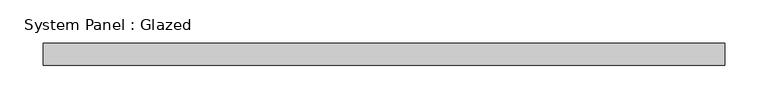
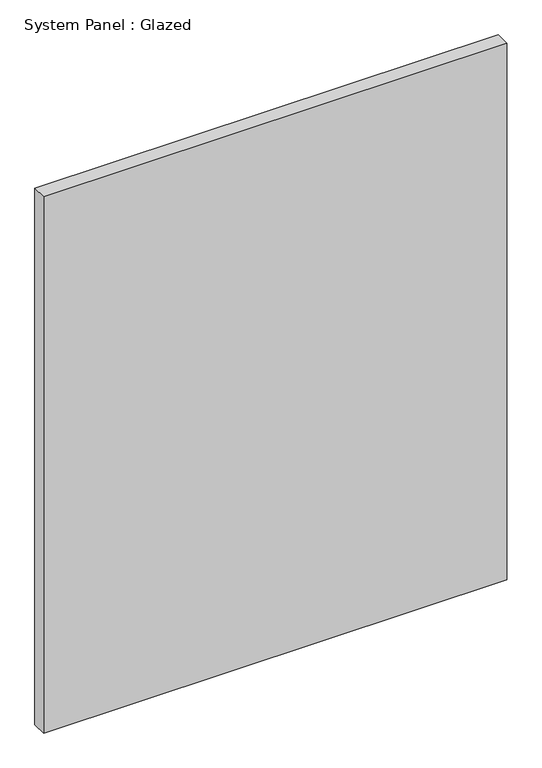
"""IFC4 building model written with IfcOpenShell, lengths in millimetres: plate geometry, System Panel : Glazed."""

from ifc_helpers import new_model, si_unit, origin, origin_with_axes, place, context, project, spatial, polyline, outline, extrude, source, transform, mapped, element, save


def system_panel_glazed_6a49b045(model_context):
    return source(origin(), model_context, "Body", "SweptSolid", [
        extrude(outline(polyline([(394.3296124, 19.05), (-394.3296124, 19.05), (-394.3296124, 44.45), (394.3296124, 44.45), (394.3296124, 19.05)])), origin_with_axes(), (0.0, 0.0, 1.0), 964.934107),
    ])


if __name__ == "__main__":
    model = new_model("IFC4")
    model_context = context("Model", 3, world=origin())
    ifc_project = project(units=[si_unit("LENGTHUNIT", "METRE", prefix="MILLI")], contexts=[model_context])
    site = spatial("IfcSite", under=ifc_project)
    building = spatial("IfcBuilding", under=site)
    placement = place(None, origin())
    system_panel_glazed_shape = system_panel_glazed_6a49b045(model_context)
    element("IfcPlate", 1, ObjectType="System Panel : Glazed", at=placement, inside=building, context=model_context, shape_type="MappedRepresentation", body=[
        mapped(system_panel_glazed_shape, transform((0.0, 0.0, 0.0), x_axis=(1.0, 0.0, 0.0), y_axis=(0.0, 1.0, 0.0), z_axis=(0.0, 0.0, 1.0))),
    ])
    save(model, "model.ifc")

# Revit data of these elements
# Type "System Panel : Glazed"
#   Construction Type Id = "GSP4R"
#   Analytic Construction = "1/8 in Pilkington single glazing"
#   Visual Light Transmittance = 0.9
#   Solar Heat Gain Coefficient = 0.86
#   Heat Transfer Coefficient (U) = 1.18115 BTU/(h·ft²·°F)
# Element 1 (IfcPlate, "System Panel : Glazed")
#   Materials on its faces: "Glass"
# Materials
#   "Glass": class "Glass", colour RGB 0 128 192, transparency 0.75, Description = "Soda Lime Glass", Cost = 0
